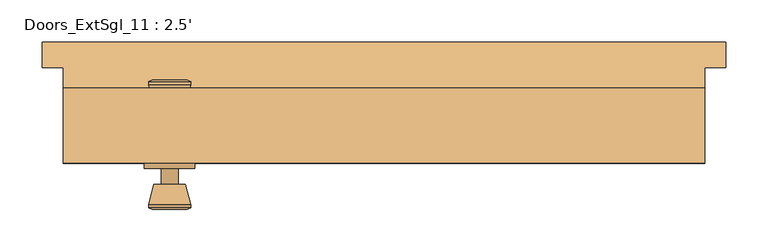
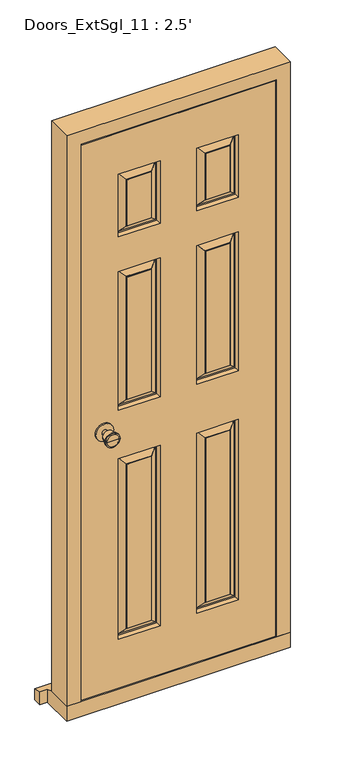
"""IFC4 building model written with IfcOpenShell, lengths in millimetres: door geometry, Doors_ExtSgl_11 : 2.5'."""

from ifc_helpers import new_model, si_unit, point, frame, frame_2d, origin, place, context, project, spatial, polyline, circle_curve, trimmed, segment, composite_curve, outline, extrude, faceted_brep, source, transform, mapped, element, save
from ifc_brep_helpers import plane_surface, cylinder_surface, revolved_surface, advanced_brep


def doors_extsgl_11_2_5_c7418333(model_context):
    return source(origin(), model_context, "Body", "SolidModel", [
        advanced_brep(
        [(-254.5, -51.42, 1000.0), (-244.5, -51.42, 1000.0), (-264.5, -51.42, 1000.0), (-234.0241324, -100.42, 1000.0), (-254.5, -100.42, 1000.0), (-274.9758676, -100.42, 1000.0), (-229.5, -98.5921319, 1000.0), (-279.5, -98.5921319, 1000.0), (-229.5, -95.1284537, 1000.0), (-279.5, -95.1284537, 1000.0), (-235.863764, -70.42, 1000.0), (-273.136236, -70.42, 1000.0), (-244.5, -70.42, 1000.0), (-264.5, -70.42, 1000.0)],
        [
            (0, 1),
            (1, 2, circle_curve(frame((-254.5, -51.42, 1000.0), z_axis=(0.0, 1.0, 0.0), x_axis=(-1.0, 0.0, 0.0)), 10.0)),
            (2, 0),
            (2, 1, circle_curve(frame((-254.5, -51.42, 1000.0), z_axis=(0.0, 1.0, 0.0), x_axis=(-1.0, 0.0, 0.0)), 10.0)),
            (3, 4),
            (4, 5),
            (5, 3, circle_curve(frame((-254.5, -100.42, 1000.0), z_axis=(0.0, -1.0, 0.0), x_axis=(-1.0, 0.0, 0.0)), 20.4758676)),
            (3, 5, circle_curve(frame((-254.5, -100.42, 1000.0), z_axis=(0.0, -1.0, 0.0), x_axis=(-1.0, 0.0, 0.0)), 20.4758676)),
            (6, 3),
            (5, 7),
            (7, 6, circle_curve(frame((-254.5, -98.5921319, 1000.0), z_axis=(0.0, -1.0, 0.0), x_axis=(-1.0, 0.0, 0.0)), 25.0)),
            (6, 7, circle_curve(frame((-254.5, -98.5921319, 1000.0), z_axis=(0.0, -1.0, 0.0), x_axis=(-1.0, 0.0, 0.0)), 25.0)),
            (8, 6),
            (7, 9),
            (9, 8, circle_curve(frame((-254.5, -95.1284537, 1000.0), z_axis=(0.0, -1.0, 0.0), x_axis=(-1.0, 0.0, 0.0)), 25.0)),
            (8, 9, circle_curve(frame((-254.5, -95.1284537, 1000.0), z_axis=(0.0, -1.0, 0.0), x_axis=(-1.0, 0.0, 0.0)), 25.0)),
            (10, 8),
            (9, 11),
            (11, 10, circle_curve(frame((-254.5, -70.42, 1000.0), z_axis=(0.0, -1.0, 0.0), x_axis=(-1.0, 0.0, 0.0)), 18.636236)),
            (10, 11, circle_curve(frame((-254.5, -70.42, 1000.0), z_axis=(0.0, -1.0, 0.0), x_axis=(-1.0, 0.0, 0.0)), 18.636236)),
            (12, 10),
            (11, 13),
            (13, 12, circle_curve(frame((-254.5, -70.42, 1000.0), z_axis=(0.0, -1.0, 0.0), x_axis=(-1.0, 0.0, 0.0)), 10.0)),
            (12, 13, circle_curve(frame((-254.5, -70.42, 1000.0), z_axis=(0.0, -1.0, 0.0), x_axis=(-1.0, 0.0, 0.0)), 10.0)),
            (1, 12),
            (13, 2),
        ],
        [
            plane_surface(frame((-254.5, -51.42, 1000.0), z_axis=(0.0, 1.0, 0.0), x_axis=(-1.0, 0.0, 0.0))),
            plane_surface(frame((-254.5, -100.42, 1000.0), z_axis=(0.0, -1.0, 0.0), x_axis=(-1.0, 0.0, 0.0))),
            revolved_surface(polyline([(-274.9758676, -100.42, 1000.0), (-279.5, -98.5921319, 1000.0)]), (-254.5, -51.42, 1000.0), (0.0, 1.0, 0.0)),
            cylinder_surface(frame((-254.5, -51.42, 1000.0), z_axis=(0.0, 1.0, 0.0), x_axis=(-1.0, 0.0, 0.0)), 25.0),
            revolved_surface(polyline([(-279.5, -95.1284537, 1000.0), (-273.136236, -70.42, 1000.0)]), (-254.5, -51.42, 1000.0), (0.0, 1.0, 0.0)),
            plane_surface(frame((-254.5, -70.42, 1000.0), z_axis=(0.0, 1.0, 0.0), x_axis=(-1.0, 0.0, 0.0))),
            cylinder_surface(frame((-254.5, -51.42, 1000.0), z_axis=(0.0, 1.0, 0.0), x_axis=(-1.0, 0.0, 0.0)), 10.0),
        ],
        [
            (0, [[1, 2, 3]]),
            (0, [[-3, 4, -1]]),
            (1, [[5, 6, 7]]),
            (1, [[-6, -5, 8]]),
            (2, [[9, -7, 10, 11]]),
            (2, [[-10, -8, -9, 12]]),
            (3, [[13, -11, 14, 15]]),
            (3, [[-14, -12, -13, 16]]),
            (4, [[17, -15, 18, 19]]),
            (4, [[-18, -16, -17, 20]]),
            (5, [[21, -19, 22, 23]]),
            (5, [[-22, -20, -21, 24]]),
            (6, [[25, -23, 26, -2]]),
            (6, [[-26, -24, -25, -4]]),
        ],
    ),
        extrude(outline(composite_curve([segment(trimmed(circle_curve(frame_2d((1000.0, -254.5)), 30.0), [point((1000.0, -284.5))], [point((1000.0, -224.5))], False, "CARTESIAN"), True, "CONTINUOUS"), segment(trimmed(circle_curve(frame_2d((1000.0, -254.5)), 30.0), [point((1000.0, -224.5))], [point((1000.0, -284.5))], False, "CARTESIAN"), True, "CONTINUOUS")], self_intersect=False)), frame((0.0, -51.42, 0.0), z_axis=(0.0, 1.0, 0.0), x_axis=(0.0, 0.0, 1.0)), (0.0, 0.0, 1.0), 6.0),
        advanced_brep(
        [(-254.5, 4.58, 1000.0), (-264.5, 4.58, 1000.0), (-244.5, 4.58, 1000.0), (-234.0241324, 53.58, 1000.0), (-274.9758676, 53.58, 1000.0), (-254.5, 53.58, 1000.0), (-229.5, 51.7521319, 1000.0), (-279.5, 51.7521319, 1000.0), (-229.5, 48.2884537, 1000.0), (-279.5, 48.2884537, 1000.0), (-235.863764, 23.58, 1000.0), (-273.136236, 23.58, 1000.0), (-244.5, 23.58, 1000.0), (-264.5, 23.58, 1000.0)],
        [
            (0, 1),
            (1, 2, circle_curve(frame((-254.5, 4.58, 1000.0), z_axis=(0.0, -1.0, 0.0), x_axis=(-1.0, 0.0, 0.0)), 10.0)),
            (2, 0),
            (2, 1, circle_curve(frame((-254.5, 4.58, 1000.0), z_axis=(0.0, -1.0, 0.0), x_axis=(-1.0, 0.0, 0.0)), 10.0)),
            (3, 4, circle_curve(frame((-254.5, 53.58, 1000.0), z_axis=(0.0, 1.0, 0.0), x_axis=(-1.0, 0.0, 0.0)), 20.4758676)),
            (4, 5),
            (5, 3),
            (4, 3, circle_curve(frame((-254.5, 53.58, 1000.0), z_axis=(0.0, 1.0, 0.0), x_axis=(-1.0, 0.0, 0.0)), 20.4758676)),
            (6, 7, circle_curve(frame((-254.5, 51.7521319, 1000.0), z_axis=(0.0, 1.0, 0.0), x_axis=(-1.0, 0.0, 0.0)), 25.0)),
            (7, 4),
            (3, 6),
            (7, 6, circle_curve(frame((-254.5, 51.7521319, 1000.0), z_axis=(0.0, 1.0, 0.0), x_axis=(-1.0, 0.0, 0.0)), 25.0)),
            (8, 9, circle_curve(frame((-254.5, 48.2884537, 1000.0), z_axis=(0.0, 1.0, 0.0), x_axis=(-1.0, 0.0, 0.0)), 25.0)),
            (9, 7),
            (6, 8),
            (9, 8, circle_curve(frame((-254.5, 48.2884537, 1000.0), z_axis=(0.0, 1.0, 0.0), x_axis=(-1.0, 0.0, 0.0)), 25.0)),
            (10, 11, circle_curve(frame((-254.5, 23.58, 1000.0), z_axis=(0.0, 1.0, 0.0), x_axis=(-1.0, 0.0, 0.0)), 18.636236)),
            (11, 9),
            (8, 10),
            (11, 10, circle_curve(frame((-254.5, 23.58, 1000.0), z_axis=(0.0, 1.0, 0.0), x_axis=(-1.0, 0.0, 0.0)), 18.636236)),
            (12, 13, circle_curve(frame((-254.5, 23.58, 1000.0), z_axis=(0.0, 1.0, 0.0), x_axis=(-1.0, 0.0, 0.0)), 10.0)),
            (13, 11),
            (10, 12),
            (13, 12, circle_curve(frame((-254.5, 23.58, 1000.0), z_axis=(0.0, 1.0, 0.0), x_axis=(-1.0, 0.0, 0.0)), 10.0)),
            (1, 13),
            (12, 2),
        ],
        [
            plane_surface(frame((-254.5, 4.58, 1000.0), z_axis=(0.0, -1.0, 0.0), x_axis=(-1.0, 0.0, 0.0))),
            plane_surface(frame((-254.5, 53.58, 1000.0), z_axis=(0.0, 1.0, 0.0), x_axis=(-1.0, 0.0, 0.0))),
            revolved_surface(polyline([(-274.9758676, 53.58, 1000.0), (-279.5, 51.7521319, 1000.0)]), (-254.5, 4.58, 1000.0), (0.0, -1.0, 0.0)),
            cylinder_surface(frame((-254.5, 4.58, 1000.0), z_axis=(0.0, -1.0, 0.0), x_axis=(-1.0, 0.0, 0.0)), 25.0),
            revolved_surface(polyline([(-279.5, 48.2884537, 1000.0), (-273.136236, 23.58, 1000.0)]), (-254.5, 4.58, 1000.0), (0.0, -1.0, 0.0)),
            plane_surface(frame((-254.5, 23.58, 1000.0), z_axis=(0.0, -1.0, 0.0), x_axis=(-1.0, 0.0, 0.0))),
            cylinder_surface(frame((-254.5, 4.58, 1000.0), z_axis=(0.0, -1.0, 0.0), x_axis=(-1.0, 0.0, 0.0)), 10.0),
        ],
        [
            (0, [[1, 2, 3]]),
            (0, [[-3, 4, -1]]),
            (1, [[5, 6, 7]]),
            (1, [[8, -7, -6]]),
            (2, [[9, 10, -5, 11]]),
            (2, [[12, -11, -8, -10]]),
            (3, [[13, 14, -9, 15]]),
            (3, [[16, -15, -12, -14]]),
            (4, [[17, 18, -13, 19]]),
            (4, [[20, -19, -16, -18]]),
            (5, [[21, 22, -17, 23]]),
            (5, [[24, -23, -20, -22]]),
            (6, [[-2, 25, -21, 26]]),
            (6, [[-4, -26, -24, -25]]),
        ],
    ),
        extrude(outline(composite_curve([segment(trimmed(circle_curve(frame_2d((1000.0, -254.5)), 30.0), [point((1000.0, -284.5))], [point((1000.0, -224.5))], False, "CARTESIAN"), True, "CONTINUOUS"), segment(trimmed(circle_curve(frame_2d((1000.0, -254.5)), 30.0), [point((1000.0, -224.5))], [point((1000.0, -284.5))], False, "CARTESIAN"), True, "CONTINUOUS")], self_intersect=False)), frame((0.0, -1.42, 0.0), z_axis=(0.0, 1.0, 0.0), x_axis=(0.0, 0.0, 1.0)), (0.0, 0.0, 1.0), 6.0),
        faceted_brep([(310.5, 43.58, 54.5), (381.0, 43.58, 54.5), (381.0, -45.42, 54.5), (332.5, -45.42, 54.5), (332.5, 1.58, 54.5), (310.5, 1.58, 54.5), (310.5, 43.58, 2039.5), (-310.5, 43.58, 2039.5), (-310.5, 43.58, 54.5), (-381.0, 43.58, 54.5), (-381.0, 43.58, 2110.0), (381.0, 43.58, 2110.0), (381.0, -45.42, 2110.0), (-381.0, -45.42, 2110.0), (-381.0, -45.42, 54.5), (-332.5, -45.42, 54.5), (-332.5, -45.42, 2061.5), (332.5, -45.42, 2061.5), (332.5, 1.58, 2061.5), (-332.5, 1.58, 2061.5), (-332.5, 1.58, 54.5), (-310.5, 1.58, 54.5), (-310.5, 1.58, 2039.5), (310.5, 1.58, 2039.5)], [[[0, 1, 2, 3, 4, 5]], [[1, 0, 6, 7, 8, 9, 10, 11]], [[2, 1, 11, 12]], [[3, 2, 12, 13, 14, 15, 16, 17]], [[4, 3, 17, 18]], [[5, 4, 18, 19, 20, 21, 22, 23]], [[0, 5, 23, 6]], [[8, 7, 22, 21]], [[9, 8, 21, 20, 15, 14]], [[10, 9, 14, 13]], [[16, 15, 20, 19]], [[11, 10, 13, 12]], [[17, 16, 19, 18]], [[7, 6, 23, 22]]]),
        faceted_brep([(329.5, -45.42, 58.5), (329.5, -45.42, 2058.5), (-330.4250294, -45.42, 2058.5), (-330.4250294, -45.42, 58.5), (-62.5, -45.42, 883.5), (-62.5, -45.42, 233.5), (-204.5, -45.42, 233.5), (-204.5, -45.42, 883.5), (204.5, -45.42, 883.5), (204.5, -45.42, 233.5), (62.5, -45.42, 233.5), (62.5, -45.42, 883.5), (-62.5, -45.42, 1558.5), (-62.5, -45.42, 1058.5), (-204.5, -45.42, 1058.5), (-204.5, -45.42, 1558.5), (204.5, -45.42, 1558.5), (204.5, -45.42, 1058.5), (62.5, -45.42, 1058.5), (62.5, -45.42, 1558.5), (-62.5, -45.42, 1908.5), (-62.5, -45.42, 1683.5), (-204.5, -45.42, 1683.5), (-204.5, -45.42, 1908.5), (62.5, -45.42, 1683.5), (62.5, -45.42, 1908.5), (204.5, -45.42, 1908.5), (204.5, -45.42, 1683.5), (-92.5, -45.42, 263.5), (-92.5, -45.42, 853.5), (-174.5, -45.42, 853.5), (-174.5, -45.42, 263.5), (174.5, -45.42, 263.5), (174.5, -45.42, 853.5), (92.5, -45.42, 853.5), (92.5, -45.42, 263.5), (-92.5, -45.42, 1088.5), (-92.5, -45.42, 1528.5), (-174.5, -45.42, 1528.5), (-174.5, -45.42, 1088.5), (174.5, -45.42, 1088.5), (174.5, -45.42, 1528.5), (92.5, -45.42, 1528.5), (92.5, -45.42, 1088.5), (-92.5, -45.42, 1713.5), (-92.5, -45.42, 1878.5), (-174.5, -45.42, 1878.5), (-174.5, -45.42, 1713.5), (92.5, -45.42, 1878.5), (92.5, -45.42, 1713.5), (174.5, -45.42, 1713.5), (174.5, -45.42, 1878.5), (329.5, -1.42, 58.5), (-330.4250294, -1.42, 58.5), (-330.4250294, -1.42, 2058.5), (329.5, -1.42, 2058.5), (62.5, -1.42, 883.5), (62.5, -1.42, 233.5), (204.5, -1.42, 233.5), (204.5, -1.42, 883.5), (-204.5, -1.42, 883.5), (-204.5, -1.42, 233.5), (-62.5, -1.42, 233.5), (-62.5, -1.42, 883.5), (62.5, -1.42, 1558.5), (62.5, -1.42, 1058.5), (204.5, -1.42, 1058.5), (204.5, -1.42, 1558.5), (-204.5, -1.42, 1558.5), (-204.5, -1.42, 1058.5), (-62.5, -1.42, 1058.5), (-62.5, -1.42, 1558.5), (62.5, -1.42, 1908.5), (62.5, -1.42, 1683.5), (204.5, -1.42, 1683.5), (204.5, -1.42, 1908.5), (-204.5, -1.42, 1908.5), (-204.5, -1.42, 1683.5), (-62.5, -1.42, 1683.5), (-62.5, -1.42, 1908.5), (92.5, -1.42, 263.5), (92.5, -1.42, 853.5), (174.5, -1.42, 853.5), (174.5, -1.42, 263.5), (-174.5, -1.42, 263.5), (-174.5, -1.42, 853.5), (-92.5, -1.42, 853.5), (-92.5, -1.42, 263.5), (92.5, -1.42, 1088.5), (92.5, -1.42, 1528.5), (174.5, -1.42, 1528.5), (174.5, -1.42, 1088.5), (-174.5, -1.42, 1088.5), (-174.5, -1.42, 1528.5), (-92.5, -1.42, 1528.5), (-92.5, -1.42, 1088.5), (92.5, -1.42, 1713.5), (92.5, -1.42, 1878.5), (174.5, -1.42, 1878.5), (174.5, -1.42, 1713.5), (-174.5, -1.42, 1713.5), (-174.5, -1.42, 1878.5), (-92.5, -1.42, 1878.5), (-92.5, -1.42, 1713.5), (65.5, -16.42, 880.5), (65.5, -16.42, 236.5), (90.5, -2.42, 855.5), (90.5, -2.42, 261.5), (70.5, -16.42, 241.5), (70.5, -16.42, 875.5), (92.5, -2.42, 263.5), (92.5, -2.42, 853.5), (201.5, -16.42, 236.5), (176.5, -2.42, 261.5), (196.5, -16.42, 241.5), (174.5, -2.42, 263.5), (201.5, -16.42, 880.5), (176.5, -2.42, 855.5), (196.5, -16.42, 875.5), (174.5, -2.42, 853.5), (-201.5, -16.42, 880.5), (-201.5, -16.42, 236.5), (-176.5, -2.42, 855.5), (-176.5, -2.42, 261.5), (-196.5, -16.42, 241.5), (-196.5, -16.42, 875.5), (-174.5, -2.42, 263.5), (-174.5, -2.42, 853.5), (-65.5, -16.42, 236.5), (-90.5, -2.42, 261.5), (-70.5, -16.42, 241.5), (-92.5, -2.42, 263.5), (-65.5, -16.42, 880.5), (-90.5, -2.42, 855.5), (-70.5, -16.42, 875.5), (-92.5, -2.42, 853.5), (-92.5, -44.42, 263.5), (-92.5, -44.42, 853.5), (-70.5, -30.42, 241.5), (-70.5, -30.42, 875.5), (-90.5, -44.42, 855.5), (-90.5, -44.42, 261.5), (-65.5, -30.42, 880.5), (-65.5, -30.42, 236.5), (-174.5, -44.42, 853.5), (-196.5, -30.42, 875.5), (-176.5, -44.42, 855.5), (-201.5, -30.42, 880.5), (-174.5, -44.42, 263.5), (-196.5, -30.42, 241.5), (-176.5, -44.42, 261.5), (-201.5, -30.42, 236.5), (201.5, -30.42, 880.5), (201.5, -30.42, 236.5), (176.5, -44.42, 855.5), (176.5, -44.42, 261.5), (196.5, -30.42, 241.5), (196.5, -30.42, 875.5), (174.5, -44.42, 263.5), (174.5, -44.42, 853.5), (65.5, -30.42, 236.5), (90.5, -44.42, 261.5), (70.5, -30.42, 241.5), (92.5, -44.42, 263.5), (65.5, -30.42, 880.5), (90.5, -44.42, 855.5), (70.5, -30.42, 875.5), (92.5, -44.42, 853.5), (92.5, -2.42, 1088.5), (92.5, -2.42, 1528.5), (70.5, -16.42, 1066.5), (70.5, -16.42, 1550.5), (90.5, -2.42, 1530.5), (90.5, -2.42, 1086.5), (65.5, -16.42, 1555.5), (65.5, -16.42, 1061.5), (174.5, -2.42, 1528.5), (196.5, -16.42, 1550.5), (176.5, -2.42, 1530.5), (201.5, -16.42, 1555.5), (174.5, -2.42, 1088.5), (196.5, -16.42, 1066.5), (176.5, -2.42, 1086.5), (201.5, -16.42, 1061.5), (-174.5, -2.42, 1088.5), (-174.5, -2.42, 1528.5), (-196.5, -16.42, 1066.5), (-196.5, -16.42, 1550.5), (-176.5, -2.42, 1530.5), (-176.5, -2.42, 1086.5), (-201.5, -16.42, 1555.5), (-201.5, -16.42, 1061.5), (-92.5, -2.42, 1528.5), (-70.5, -16.42, 1550.5), (-90.5, -2.42, 1530.5), (-65.5, -16.42, 1555.5), (-92.5, -2.42, 1088.5), (-70.5, -16.42, 1066.5), (-90.5, -2.42, 1086.5), (-65.5, -16.42, 1061.5), (-92.5, -44.42, 1088.5), (-92.5, -44.42, 1528.5), (-70.5, -30.42, 1066.5), (-70.5, -30.42, 1550.5), (-90.5, -44.42, 1530.5), (-90.5, -44.42, 1086.5), (-65.5, -30.42, 1555.5), (-65.5, -30.42, 1061.5), (-174.5, -44.42, 1528.5), (-196.5, -30.42, 1550.5), (-176.5, -44.42, 1530.5), (-201.5, -30.42, 1555.5), (-174.5, -44.42, 1088.5), (-196.5, -30.42, 1066.5), (-176.5, -44.42, 1086.5), (-201.5, -30.42, 1061.5), (201.5, -30.42, 1555.5), (201.5, -30.42, 1061.5), (176.5, -44.42, 1530.5), (176.5, -44.42, 1086.5), (196.5, -30.42, 1066.5), (196.5, -30.42, 1550.5), (174.5, -44.42, 1088.5), (174.5, -44.42, 1528.5), (65.5, -30.42, 1061.5), (90.5, -44.42, 1086.5), (70.5, -30.42, 1066.5), (92.5, -44.42, 1088.5), (65.5, -30.42, 1555.5), (90.5, -44.42, 1530.5), (70.5, -30.42, 1550.5), (92.5, -44.42, 1528.5), (92.5, -2.42, 1713.5), (92.5, -2.42, 1878.5), (70.5, -16.42, 1691.5), (70.5, -16.42, 1900.5), (90.5, -2.42, 1880.5), (90.5, -2.42, 1711.5), (65.5, -16.42, 1905.5), (65.5, -16.42, 1686.5), (174.5, -2.42, 1878.5), (196.5, -16.42, 1900.5), (176.5, -2.42, 1880.5), (201.5, -16.42, 1905.5), (174.5, -2.42, 1713.5), (196.5, -16.42, 1691.5), (176.5, -2.42, 1711.5), (201.5, -16.42, 1686.5), (-174.5, -2.42, 1713.5), (-174.5, -2.42, 1878.5), (-196.5, -16.42, 1691.5), (-196.5, -16.42, 1900.5), (-176.5, -2.42, 1880.5), (-176.5, -2.42, 1711.5), (-201.5, -16.42, 1905.5), (-201.5, -16.42, 1686.5), (-92.5, -2.42, 1878.5), (-70.5, -16.42, 1900.5), (-90.5, -2.42, 1880.5), (-65.5, -16.42, 1905.5), (-92.5, -2.42, 1713.5), (-70.5, -16.42, 1691.5), (-90.5, -2.42, 1711.5), (-65.5, -16.42, 1686.5), (-92.5, -44.42, 1713.5), (-92.5, -44.42, 1878.5), (-70.5, -30.42, 1691.5), (-70.5, -30.42, 1900.5), (-90.5, -44.42, 1880.5), (-90.5, -44.42, 1711.5), (-65.5, -30.42, 1905.5), (-65.5, -30.42, 1686.5), (-174.5, -44.42, 1878.5), (-196.5, -30.42, 1900.5), (-176.5, -44.42, 1880.5), (-201.5, -30.42, 1905.5), (-174.5, -44.42, 1713.5), (-196.5, -30.42, 1691.5), (-176.5, -44.42, 1711.5), (-201.5, -30.42, 1686.5), (92.5, -44.42, 1878.5), (92.5, -44.42, 1713.5), (70.5, -30.42, 1900.5), (70.5, -30.42, 1691.5), (90.5, -44.42, 1711.5), (90.5, -44.42, 1880.5), (65.5, -30.42, 1686.5), (65.5, -30.42, 1905.5), (174.5, -44.42, 1713.5), (196.5, -30.42, 1691.5), (176.5, -44.42, 1711.5), (201.5, -30.42, 1686.5), (174.5, -44.42, 1878.5), (196.5, -30.42, 1900.5), (176.5, -44.42, 1880.5), (201.5, -30.42, 1905.5)], [[[0, 1, 2, 3], [4, 5, 6, 7], [8, 9, 10, 11], [12, 13, 14, 15], [16, 17, 18, 19], [20, 21, 22, 23], [24, 25, 26, 27]], [[28, 29, 30, 31]], [[32, 33, 34, 35]], [[36, 37, 38, 39]], [[40, 41, 42, 43]], [[44, 45, 46, 47]], [[48, 49, 50, 51]], [[52, 53, 54, 55], [56, 57, 58, 59], [60, 61, 62, 63], [64, 65, 66, 67], [68, 69, 70, 71], [72, 73, 74, 75], [76, 77, 78, 79]], [[80, 81, 82, 83]], [[84, 85, 86, 87]], [[88, 89, 90, 91]], [[92, 93, 94, 95]], [[96, 97, 98, 99]], [[100, 101, 102, 103]], [[1, 0, 52, 55]], [[2, 1, 55, 54]], [[3, 2, 54, 53]], [[0, 3, 53, 52]], [[104, 105, 57, 56]], [[106, 107, 108, 109]], [[80, 110, 111, 81]], [[57, 105, 112, 58]], [[108, 107, 113, 114]], [[110, 80, 83, 115]], [[58, 112, 116, 59]], [[114, 113, 117, 118]], [[115, 83, 82, 119]], [[104, 56, 59, 116]], [[105, 104, 116, 112], [109, 108, 114, 118]], [[106, 109, 118, 117]], [[107, 106, 117, 113], [111, 110, 115, 119]], [[81, 111, 119, 82]], [[120, 121, 61, 60]], [[122, 123, 124, 125]], [[84, 126, 127, 85]], [[61, 121, 128, 62]], [[124, 123, 129, 130]], [[126, 84, 87, 131]], [[62, 128, 132, 63]], [[130, 129, 133, 134]], [[131, 87, 86, 135]], [[120, 60, 63, 132]], [[121, 120, 132, 128], [125, 124, 130, 134]], [[122, 125, 134, 133]], [[123, 122, 133, 129], [127, 126, 131, 135]], [[85, 127, 135, 86]], [[136, 137, 29, 28]], [[138, 139, 140, 141]], [[4, 142, 143, 5]], [[29, 137, 144, 30]], [[140, 139, 145, 146]], [[142, 4, 7, 147]], [[30, 144, 148, 31]], [[146, 145, 149, 150]], [[147, 7, 6, 151]], [[136, 28, 31, 148]], [[141, 140, 146, 150], [137, 136, 148, 144]], [[138, 141, 150, 149]], [[143, 142, 147, 151], [139, 138, 149, 145]], [[5, 143, 151, 6]], [[152, 153, 9, 8]], [[154, 155, 156, 157]], [[32, 158, 159, 33]], [[9, 153, 160, 10]], [[156, 155, 161, 162]], [[158, 32, 35, 163]], [[10, 160, 164, 11]], [[162, 161, 165, 166]], [[163, 35, 34, 167]], [[152, 8, 11, 164]], [[153, 152, 164, 160], [157, 156, 162, 166]], [[154, 157, 166, 165]], [[155, 154, 165, 161], [159, 158, 163, 167]], [[33, 159, 167, 34]], [[168, 169, 89, 88]], [[170, 171, 172, 173]], [[64, 174, 175, 65]], [[89, 169, 176, 90]], [[172, 171, 177, 178]], [[174, 64, 67, 179]], [[90, 176, 180, 91]], [[178, 177, 181, 182]], [[179, 67, 66, 183]], [[168, 88, 91, 180]], [[173, 172, 178, 182], [169, 168, 180, 176]], [[170, 173, 182, 181]], [[175, 174, 179, 183], [171, 170, 181, 177]], [[65, 175, 183, 66]], [[184, 185, 93, 92]], [[186, 187, 188, 189]], [[68, 190, 191, 69]], [[93, 185, 192, 94]], [[188, 187, 193, 194]], [[190, 68, 71, 195]], [[94, 192, 196, 95]], [[194, 193, 197, 198]], [[195, 71, 70, 199]], [[184, 92, 95, 196]], [[189, 188, 194, 198], [185, 184, 196, 192]], [[186, 189, 198, 197]], [[191, 190, 195, 199], [187, 186, 197, 193]], [[69, 191, 199, 70]], [[200, 201, 37, 36]], [[202, 203, 204, 205]], [[12, 206, 207, 13]], [[37, 201, 208, 38]], [[204, 203, 209, 210]], [[206, 12, 15, 211]], [[38, 208, 212, 39]], [[210, 209, 213, 214]], [[211, 15, 14, 215]], [[200, 36, 39, 212]], [[205, 204, 210, 214], [201, 200, 212, 208]], [[202, 205, 214, 213]], [[207, 206, 211, 215], [203, 202, 213, 209]], [[13, 207, 215, 14]], [[216, 217, 17, 16]], [[218, 219, 220, 221]], [[40, 222, 223, 41]], [[17, 217, 224, 18]], [[220, 219, 225, 226]], [[222, 40, 43, 227]], [[18, 224, 228, 19]], [[226, 225, 229, 230]], [[227, 43, 42, 231]], [[216, 16, 19, 228]], [[217, 216, 228, 224], [221, 220, 226, 230]], [[218, 221, 230, 229]], [[219, 218, 229, 225], [223, 222, 227, 231]], [[41, 223, 231, 42]], [[232, 233, 97, 96]], [[234, 235, 236, 237]], [[72, 238, 239, 73]], [[97, 233, 240, 98]], [[236, 235, 241, 242]], [[238, 72, 75, 243]], [[98, 240, 244, 99]], [[242, 241, 245, 246]], [[243, 75, 74, 247]], [[232, 96, 99, 244]], [[237, 236, 242, 246], [233, 232, 244, 240]], [[234, 237, 246, 245]], [[239, 238, 243, 247], [235, 234, 245, 241]], [[73, 239, 247, 74]], [[248, 249, 101, 100]], [[250, 251, 252, 253]], [[76, 254, 255, 77]], [[101, 249, 256, 102]], [[252, 251, 257, 258]], [[254, 76, 79, 259]], [[102, 256, 260, 103]], [[258, 257, 261, 262]], [[259, 79, 78, 263]], [[248, 100, 103, 260]], [[253, 252, 258, 262], [249, 248, 260, 256]], [[250, 253, 262, 261]], [[255, 254, 259, 263], [251, 250, 261, 257]], [[77, 255, 263, 78]], [[264, 265, 45, 44]], [[266, 267, 268, 269]], [[20, 270, 271, 21]], [[45, 265, 272, 46]], [[268, 267, 273, 274]], [[270, 20, 23, 275]], [[46, 272, 276, 47]], [[274, 273, 277, 278]], [[275, 23, 22, 279]], [[264, 44, 47, 276]], [[269, 268, 274, 278], [265, 264, 276, 272]], [[266, 269, 278, 277]], [[271, 270, 275, 279], [267, 266, 277, 273]], [[21, 271, 279, 22]], [[280, 281, 49, 48]], [[282, 283, 284, 285]], [[24, 286, 287, 25]], [[49, 281, 288, 50]], [[284, 283, 289, 290]], [[286, 24, 27, 291]], [[50, 288, 292, 51]], [[290, 289, 293, 294]], [[291, 27, 26, 295]], [[280, 48, 51, 292]], [[285, 284, 290, 294], [281, 280, 292, 288]], [[282, 285, 294, 293]], [[287, 286, 291, 295], [283, 282, 293, 289]], [[25, 287, 295, 26]]]),
        faceted_brep([(406.0, 98.58, 0.0), (406.0, 98.58, 38.5947221), (406.0, 68.58, 47.2703282), (406.0, 68.58, 0.0), (-406.0, 98.58, 38.5947221), (-406.0, 98.58, 0.0), (-406.0, 68.58, 0.0), (-406.0, 68.58, 47.2703282), (381.0, 68.58, 0.0), (381.0, -45.42, 0.0), (-381.0, -45.42, 0.0), (-381.0, 68.58, 0.0), (-381.0, 68.58, 47.2703282), (-381.0, 43.58, 54.5), (381.0, 43.58, 54.5), (381.0, 68.58, 47.2703282), (-381.0, -45.42, 54.5), (381.0, -45.42, 54.5)], [[[0, 1, 2, 3]], [[4, 5, 6, 7]], [[5, 0, 3, 8, 9, 10, 11, 6]], [[1, 0, 5, 4]], [[1, 4, 7, 12, 13, 14, 15, 2]], [[13, 16, 17, 14]], [[16, 10, 9, 17]], [[12, 11, 10, 16, 13]], [[11, 12, 7, 6]], [[8, 15, 14, 17, 9]], [[15, 8, 3, 2]]]),
    ])


if __name__ == "__main__":
    model = new_model("IFC4")
    model_context = context("Model", 3, world=origin())
    ifc_project = project(units=[si_unit("LENGTHUNIT", "METRE", prefix="MILLI")], contexts=[model_context])
    site = spatial("IfcSite", under=ifc_project)
    building = spatial("IfcBuilding", under=site)
    placement = place(None, origin())
    doors_extsgl_11_2_5_shape = doors_extsgl_11_2_5_c7418333(model_context)
    element("IfcDoor", 1, ObjectType="Doors_ExtSgl_11 : 2.5'", at=placement, inside=building, context=model_context, shape_type="MappedRepresentation", body=[
        mapped(doors_extsgl_11_2_5_shape, transform((0.0, 0.0, 0.0), x_axis=(1.0, 0.0, 0.0), y_axis=(0.0, 1.0, 0.0), z_axis=(0.0, 0.0, 1.0))),
    ])
    save(model, "model.ifc")

# Revit data of these elements
# Type "Doors_ExtSgl_11 : 2.5'"
#   Type Mark = "50"
#   Type Comments = "External Single"
#   Operation = "SingleSwingRight"
#   Construction Type Id = "MDOOR"
#   Keynote = "L20"
#   Analytic Construction = "Metal"
#   Wrap Layers (Int) from Ext = 177.5 mm
#   Wrap Layers (Ext) from Ext = 102.5 mm
#   Thickness = 44 mm
#   Stile Top of Lock rail = 1000 mm
#   Stile Top of Frieze Rail = 1625 mm
#   Stile Top Rail = 150 mm
#   Stile Shutting = 125 mm
#   Stile Muntin Rail = 125 mm
#   Stile Lock Rail = 175 mm
#   Stile Intermediate/Frieze = 125 mm
#   Stile Hanging = 125 mm
#   Stile Bottom Rail = 175 mm
#   Rough Width = 762 mm
#   Rough Height = 2110 mm
#   O/A Frame Width = 64 mm
#   Heat Transfer Coefficient (U) = 3.7021 W/(m²·K)
#   Handle Z Distance = 1000 mm
#   Glazing Thickness = 24 mm
#   FrameWidth = 42 mm
#   FrameOffset - External = 25 mm
#   FrameDepth = 89 mm
#   Door Panel Width = 659 mm
#   Door Panel Thickness = 44 mm
#   Door Panel Height = 2000 mm
#   Cill Thickness = 54.5 mm
#   Handle X Distance = 75 mm
#   Height = 2110 mm
#   Structural Tolerance = 6.5 mm
#   Tolerance = 3 mm
#   Undercut = 4 mm
#   Width = 762 mm
#   Cill Projection = 30 mm
#   Cill Extension = 25 mm
#   Cavity Closer Width = 50 mm
#   Cavity Closer Offset from Ext = 102.5 mm
#   Cavity Closer Depth = 85 mm
#   Vis - Ironmongery = yes
#   Vis - Cavity Closers = yes
#   Define Thermal Properties by = 1
#   Function = 1
#   Material Door = Door - Panel
#   Material Frame = Door - Frame/Mullion
#   Material Ironmongery = Door - Handle
#   Visual Light Transmittance = 0
#   Solar Heat Gain Coefficient = 0
#   Wall Closure = (empty or 0)
# Element 1 (IfcDoor, "Doors_ExtSgl_11 : 2.5'")
#   Materials on its faces: "Door - Panel", "Door - Handle", "Door - Frame/Mullion"
# Materials
#   "Door - Panel": class "Wood", colour RGB 210 159 95, transparency 0, Keynote = "L20", Cost = 0
#   "Door - Frame/Mullion": class "Wood", colour RGB 212 179 113, transparency 0, Keynote = "L20", Cost = 0
#   "Door - Handle": colour RGB 0 0 0, transparency 0, Keynote = "P21", Cost = 0
